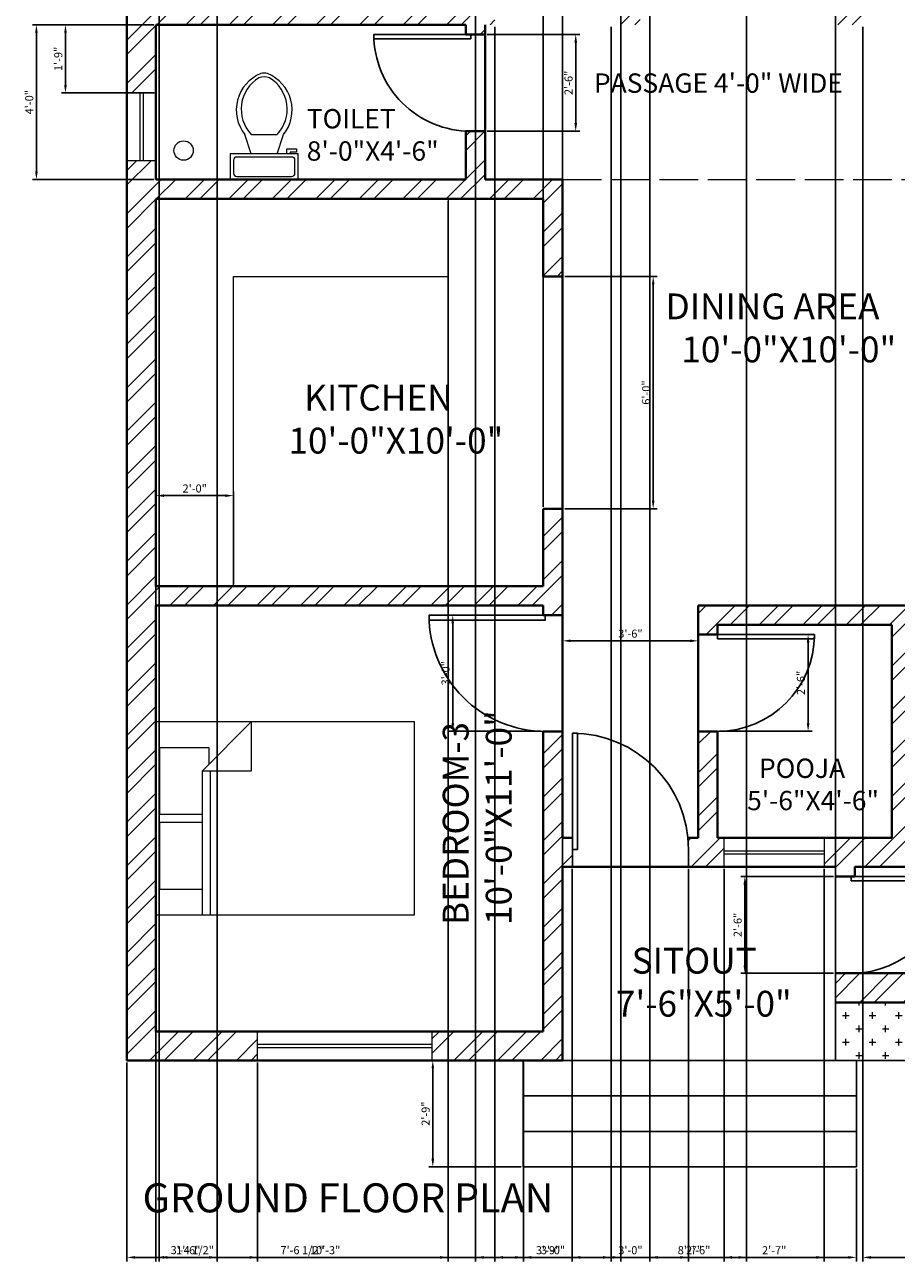
# Model space of a CAD drawing. Units: inches. Extents: x 201 to 622, y 55 to 632.
# Tile 1 of 3: x 201 to 471, y 55 to 439. Entities that reach past the tile are written whole.
import ezdxf

# ---------------------------------------------------------------- set-up
doc = ezdxf.new("R2010")
doc.units = ezdxf.units.IN
doc.linetypes.add('ACAD_ISO02W100', pattern=[15, 12, -3])
for name, color, linetype, lineweight in [('A-ANNO-DIMS', 2, 'Continuous', 18), ('A-ANNO-TITL', 7, 'Continuous', 25), ('A-AREA-IDEN', 7, 'Continuous', 18), ('A-DOOR', 4, 'Continuous', 25), ('A-FLOR', 7, 'Continuous', 25), ('A-FLOR-CASE', 8, 'Continuous', 18), ('A-FLOR-FIXT', 8, 'Continuous', 18), ('A-FLOR-OVHD', 7, 'ACAD_ISO02W100', 18), ('A-FLOR-STRS', 7, 'Continuous', 25), ('A-WALL', 7, 'Continuous', 40), ('A-WALL-PATT', 252, 'Continuous', 13)]:
    doc.layers.add(name, color=color, linetype=linetype, lineweight=lineweight)
for name, color, linetype, lineweight, true_color in [('A-FLOR-PATT', 116, 'Continuous', 13, 0x136734), ('A-FURN', 152, 'Continuous', 18, 0x2776bb), ('A-GLAZ', 152, 'Continuous', 18, 0x2776bb)]:
    doc.layers.add(name, color=color, linetype=linetype, lineweight=lineweight, true_color=true_color)
doc.styles.get("Standard").update_dxf_attribs({"font": 'arial.ttf'})
doc.dimstyles.new('ISO-25', dxfattribs={"dimtxt": 2.5, "dimasz": 2.5, "dimexe": 1.25, "dimexo": 0.625, "dimtad": 1, "dimlunit": 3, "dimtxsty": 'Standard', "dimcen": 2.5, "dimadec": 0, "dimazin": 0, "dimtfac": 1, "dimtmove": 0, "dimatfit": 3, "dimfxl": 1, "dimarcsym": 0})

# ---------------------------------------------------------------- blocks, each defined once
blk = doc.blocks.new('*U3')
for p, q in [((0, 0), (0, -6)), ((40, 0), (40, -6))]:
    blk.add_line(p, q)
blk.add_lwpolyline([(0, 0), (0, 40), (1.75, 40), (1.75, 0)], close=True)
blk.add_arc((0, 0), 40, 0, 90)
blk = doc.blocks.new('*U5')
for p, q in [((0, 0), (0, 6)), ((40, 0), (40, 6))]:
    blk.add_line(p, q)
blk.add_lwpolyline([(0, 0), (0, -40), (1.75, -40), (1.75, 0)], close=True)
blk.add_arc((0, 0), 40, 270, 0)
blk = doc.blocks.new('*U6')
for p, q in [((0, 0), (0, -6)), ((40, 0), (40, -6))]:
    blk.add_line(p, q)
blk.add_lwpolyline([(0, 0), (0, 40), (1.75, 40), (1.75, 0)], close=True)
blk.add_arc((0, 0), 40, 0, 90)
blk = doc.blocks.new('Bed - Queen')
for p, q in [((0, -80.00003), (0, 0)), ((0, 0), (59.99999, 0)), ((59.99999, 0), (59.99999, -80.00003)), ((7.99999, -1.2), (28.79998, -1.2)), ((7.99999, -14.4), (7.99999, -1.2)), ((28.79998, -1.2), (28.79998, -14.4)), ((31.19999, -1.2), (51.99999, -1.2)), ((31.19999, -14.4), (31.19999, -1.2)), ((51.99999, -1.2), (51.99999, -16.4)), ((0, -14.4), (44.8, -14.4)), ((59.99999, -29.6), (44.8, -14.4)), ((44.8, -14.4), (44.8, -29.6)), ((44.8, -16.8), (0, -16.8)), ((51.99999, -16.4), (46.79936, -16.4)), ((44.8, -29.6), (59.99999, -29.6)), ((59.99999, -80.00003), (0, -80.00003))]:
    blk.add_line(p, q)
blk = doc.blocks.new('*U9')
for p, q in [((9.5, -6), (9.5, -2)), ((-10, -8.5), (-8, -8.5)), ((-10, -9.5), (-10, -8.5)), ((-7, -9.5), (-10, -9.5)), ((-8, -8.5), (-8, -8)), ((-7, -8), (-7, -9.5)), ((-4, -8), (-6, -14)), ((4, -8), (6, -14)), ((4, -14), (-4, -14))]:
    blk.add_line(p, q)
blk.add_lwpolyline([(10.5, -8), (10.5, 0), (-10.5, 0), (-10.5, -8)], close=True)
for points in [[(-9.5, -2), (-9.5, -6)], [(8.5, -1), (-8.5, -1)], [(-8.5, -7), (8.5, -7)]]:
    blk.add_lwpolyline(points)
for centre, radius, start, end in [((-8.62, -1.88), 0.884, 81.8699, 188.1301), ((8.62, -1.88), 0.884, 351.8699, 98.1301), ((-8.62, -6.12), 0.884, 171.8699, 278.1301), ((8.62, -6.12), 0.884, 261.8699, 8.1301), ((3.52, -21.58), 12.17, 141.4691, 247.9714), ((4.2, -21.82), 11.33, 136.3677, 238.9468), ((-3.52, -21.58), 12.17, 292.0284, 38.5307), ((-4.2, -21.82), 11.33, 301.053, 43.6321), ((0, -27.88), 4, 245.7318, 294.2682), ((0, -29), 4, 254.8605, 285.1395)]:
    blk.add_arc(centre, radius, start, end)
blk = doc.blocks.new('WIN-54')
for p, q in [((0, 5), (54, 5)), ((0, 4), (54, 4))]:
    blk.add_line(p, q)
blk.add_lwpolyline([(0, 9), (54, 9), (54, 0), (0, 0)], close=True)
blk = doc.blocks.new('WIN-21')
for p, q in [((0, 5), (21, 5)), ((0, 4), (21, 4))]:
    blk.add_line(p, q)
blk.add_lwpolyline([(0, 0), (0, 9), (21, 9), (21, 0)], close=True)
blk = doc.blocks.new('*D23')
at = {"layer": 'A-ANNO-DIMS', "color": 0, "lineweight": -2, "transparency": 16777216}
for p, q in [((354.55, 118.15), (325.88, 118.15)), ((327.13, 87.65), (327.13, 115.65)), ((354.55, 85.15), (325.88, 85.15))]:
    blk.add_line(p, q, dxfattribs=at)
at = {"layer": 'A-ANNO-DIMS', "color": 0, "transparency": 16777216}
for points in [[(326.71, 115.65), (327.54, 115.65), (327.13, 118.15)], [(326.71, 87.65), (327.54, 87.65), (327.13, 85.15)]]:
    blk.add_solid(points, dxfattribs=at)
at = {"layer": 'Defpoints', "color": 0, "transparency": 16777216}
for p in [(327.13, 118.15), (355.18, 118.15), (355.18, 85.15)]:
    blk.add_point(p, dxfattribs=at)
at = {"layer": 'A-ANNO-DIMS', "color": 0, "transparency": 16777216, "insert": (325.22, 101.65), "char_height": 2.5, "attachment_point": 5, "rotation": 90}
blk.add_mtext('2\'-9"', dxfattribs=at)
blk = doc.blocks.new('*D24')
at = {"layer": 'A-ANNO-DIMS', "color": 0, "lineweight": -2, "transparency": 16777216}
for p, q in [((355.18, 84.52), (355.18, 55.85)), ((458.38, 84.52), (458.38, 55.85)), ((357.68, 57.1), (455.88, 57.1))]:
    blk.add_line(p, q, dxfattribs=at)
at = {"layer": 'A-ANNO-DIMS', "color": 0, "transparency": 16777216}
for points in [[(357.68, 57.51), (357.68, 56.68), (355.18, 57.1)], [(455.88, 57.51), (455.88, 56.68), (458.38, 57.1)]]:
    blk.add_solid(points, dxfattribs=at)
at = {"layer": 'Defpoints', "color": 0, "transparency": 16777216}
for p in [(355.18, 85.15), (458.38, 85.15), (458.38, 57.1)]:
    blk.add_point(p, dxfattribs=at)
at = {"layer": 'A-ANNO-DIMS', "color": 0, "transparency": 16777216, "insert": (406.78, 59), "char_height": 2.5, "attachment_point": 5}
blk.add_mtext('8\'-7"', dxfattribs=at)
blk = doc.blocks.new('*D25')
at = {"layer": 'A-ANNO-DIMS', "color": 0, "lineweight": -2, "transparency": 16777216}
for p, q in [((232.36, 117.52), (232.36, 55.85)), ((355.18, 117.52), (355.18, 55.85)), ((234.86, 57.1), (352.68, 57.1))]:
    blk.add_line(p, q, dxfattribs=at)
at = {"layer": 'A-ANNO-DIMS', "color": 0, "transparency": 16777216}
for points in [[(234.86, 57.51), (234.86, 56.68), (232.36, 57.1)], [(352.68, 57.51), (352.68, 56.68), (355.18, 57.1)]]:
    blk.add_solid(points, dxfattribs=at)
at = {"layer": 'Defpoints', "color": 0, "transparency": 16777216}
for p in [(232.36, 118.15), (355.18, 118.15), (355.18, 57.1)]:
    blk.add_point(p, dxfattribs=at)
at = {"layer": 'A-ANNO-DIMS', "color": 0, "transparency": 16777216, "insert": (293.77, 59), "char_height": 2.5, "attachment_point": 5}
blk.add_mtext('10\'-3"', dxfattribs=at)
blk = doc.blocks.new('*D27')
at = {"layer": 'A-ANNO-DIMS', "color": 0, "lineweight": -2, "transparency": 16777216}
for p, q in [((358.86, 626.2), (356.36, 626.2)), ((361.36, 289.77), (361.36, 627.45)), ((361.36, 626.2), (367.36, 626.2)), ((367.36, 289.77), (367.36, 627.45)), ((369.86, 626.2), (380.26, 626.2))]:
    blk.add_line(p, q, dxfattribs=at)
at = {"layer": 'A-ANNO-DIMS', "color": 0, "transparency": 16777216}
for points in [[(358.86, 626.61), (358.86, 625.78), (361.36, 626.2)], [(369.86, 626.61), (369.86, 625.78), (367.36, 626.2)]]:
    blk.add_solid(points, dxfattribs=at)
at = {"layer": 'Defpoints', "color": 0, "transparency": 16777216}
for p in [(367.36, 626.2), (361.36, 289.15), (367.36, 289.15)]:
    blk.add_point(p, dxfattribs=at)
at = {"layer": 'A-ANNO-DIMS', "color": 0, "transparency": 16777216, "insert": (376.31, 628.1), "char_height": 2.5, "attachment_point": 5}
blk.add_mtext('0\'-6"', dxfattribs=at)
blk = doc.blocks.new('*D28')
at = {"layer": 'A-ANNO-DIMS', "color": 0, "lineweight": -2, "transparency": 16777216}
for p, q in [((367.99, 361.15), (396.66, 361.15)), ((395.41, 358.65), (395.41, 291.65)), ((367.99, 289.15), (396.66, 289.15))]:
    blk.add_line(p, q, dxfattribs=at)
at = {"layer": 'A-ANNO-DIMS', "color": 0, "transparency": 16777216}
for points in [[(395, 358.65), (395.83, 358.65), (395.41, 361.15)], [(395, 291.65), (395.83, 291.65), (395.41, 289.15)]]:
    blk.add_solid(points, dxfattribs=at)
at = {"layer": 'Defpoints', "color": 0, "transparency": 16777216}
for p in [(367.36, 361.15), (367.36, 289.15), (395.41, 289.15)]:
    blk.add_point(p, dxfattribs=at)
at = {"layer": 'A-ANNO-DIMS', "color": 0, "transparency": 16777216, "insert": (393.51, 325.15), "char_height": 2.5, "attachment_point": 5, "rotation": 90}
blk.add_mtext('6\'-0"', dxfattribs=at)
blk = doc.blocks.new('*D29')
at = {"layer": 'A-ANNO-DIMS', "color": 0, "lineweight": -2, "transparency": 16777216}
for p, q in [((340.36, 588.52), (340.36, 55.85)), ((385.36, 588.52), (385.36, 55.85)), ((342.86, 57.1), (382.86, 57.1))]:
    blk.add_line(p, q, dxfattribs=at)
at = {"layer": 'A-ANNO-DIMS', "color": 0, "transparency": 16777216}
for points in [[(342.86, 57.51), (342.86, 56.68), (340.36, 57.1)], [(382.86, 57.51), (382.86, 56.68), (385.36, 57.1)]]:
    blk.add_solid(points, dxfattribs=at)
at = {"layer": 'Defpoints', "color": 0, "transparency": 16777216}
for p in [(340.36, 589.15), (385.36, 589.15), (385.36, 57.1)]:
    blk.add_point(p, dxfattribs=at)
at = {"layer": 'A-ANNO-DIMS', "color": 0, "transparency": 16777216, "insert": (362.86, 59), "char_height": 2.5, "attachment_point": 5}
blk.add_mtext('3\'-9"', dxfattribs=at)
blk = doc.blocks.new('*D35')
at = {"layer": 'A-ANNO-DIMS', "color": 0, "lineweight": -2, "transparency": 16777216}
for p, q in [((232.36, 117.52), (232.36, 55.85)), ((272.86, 117.52), (272.86, 55.85)), ((234.86, 57.1), (270.36, 57.1))]:
    blk.add_line(p, q, dxfattribs=at)
at = {"layer": 'A-ANNO-DIMS', "color": 0, "transparency": 16777216}
for points in [[(234.86, 57.51), (234.86, 56.68), (232.36, 57.1)], [(270.36, 57.51), (270.36, 56.68), (272.86, 57.1)]]:
    blk.add_solid(points, dxfattribs=at)
at = {"layer": 'Defpoints', "color": 0, "transparency": 16777216}
for p in [(232.36, 118.15), (272.86, 118.15), (272.86, 57.1)]:
    blk.add_point(p, dxfattribs=at)
at = {"layer": 'A-ANNO-DIMS', "color": 0, "transparency": 16777216, "insert": (252.61, 59.02), "char_height": 2.5, "attachment_point": 5}
blk.add_mtext('3\'-4 1/2"', dxfattribs=at)
blk = doc.blocks.new('*D37')
at = {"layer": 'A-ANNO-DIMS', "color": 0, "lineweight": -2, "transparency": 16777216}
for p, q in [((240.74, 439.15), (212.06, 439.15)), ((213.31, 420.5), (213.31, 436.65)), ((240.74, 418), (212.06, 418))]:
    blk.add_line(p, q, dxfattribs=at)
at = {"layer": 'A-ANNO-DIMS', "color": 0, "transparency": 16777216}
for points in [[(212.9, 436.65), (213.73, 436.65), (213.31, 439.15)], [(212.9, 420.5), (213.73, 420.5), (213.31, 418)]]:
    blk.add_solid(points, dxfattribs=at)
at = {"layer": 'Defpoints', "color": 0, "transparency": 16777216}
for p in [(213.31, 439.15), (241.36, 439.15), (241.36, 418)]:
    blk.add_point(p, dxfattribs=at)
at = {"layer": 'A-ANNO-DIMS', "color": 0, "transparency": 16777216, "insert": (211.41, 428.57), "char_height": 2.5, "attachment_point": 5, "rotation": 90}
blk.add_mtext('1\'-9"', dxfattribs=at)
blk = doc.blocks.new('*D38')
at = {"layer": 'A-ANNO-DIMS', "color": 0, "lineweight": -2, "transparency": 16777216}
for p, q in [((370.36, 177.52), (370.36, 55.85)), ((406.36, 177.52), (406.36, 55.85)), ((372.86, 57.1), (403.86, 57.1))]:
    blk.add_line(p, q, dxfattribs=at)
at = {"layer": 'A-ANNO-DIMS', "color": 0, "transparency": 16777216}
for points in [[(372.86, 57.51), (372.86, 56.68), (370.36, 57.1)], [(403.86, 57.51), (403.86, 56.68), (406.36, 57.1)]]:
    blk.add_solid(points, dxfattribs=at)
at = {"layer": 'Defpoints', "color": 0, "transparency": 16777216}
for p in [(370.36, 178.15), (406.36, 178.15), (406.36, 57.1)]:
    blk.add_point(p, dxfattribs=at)
at = {"layer": 'A-ANNO-DIMS', "color": 0, "transparency": 16777216, "insert": (388.36, 59), "char_height": 2.5, "attachment_point": 5}
blk.add_mtext('3\'-0"', dxfattribs=at)
blk = doc.blocks.new('*D39')
at = {"layer": 'A-ANNO-DIMS', "color": 0, "lineweight": -2, "transparency": 16777216}
for p, q in [((346.36, 438.52), (346.36, 55.85)), ((382.36, 438.52), (382.36, 55.85)), ((348.86, 57.1), (379.86, 57.1))]:
    blk.add_line(p, q, dxfattribs=at)
at = {"layer": 'A-ANNO-DIMS', "color": 0, "transparency": 16777216}
for points in [[(348.86, 57.51), (348.86, 56.68), (346.36, 57.1)], [(379.86, 57.51), (379.86, 56.68), (382.36, 57.1)]]:
    blk.add_solid(points, dxfattribs=at)
at = {"layer": 'Defpoints', "color": 0, "transparency": 16777216}
for p in [(346.36, 439.15), (382.36, 439.15), (382.36, 57.1)]:
    blk.add_point(p, dxfattribs=at)
at = {"layer": 'A-ANNO-DIMS', "color": 0, "transparency": 16777216, "insert": (364.36, 59), "char_height": 2.5, "attachment_point": 5}
blk.add_mtext('3\'-0"', dxfattribs=at)
blk = doc.blocks.new('*D40')
at = {"layer": 'A-ANNO-DIMS', "color": 0, "lineweight": -2, "transparency": 16777216}
for p, q in [((394.36, 486.52), (394.36, 55.85)), ((424.36, 486.52), (424.36, 55.85)), ((396.86, 57.1), (421.86, 57.1))]:
    blk.add_line(p, q, dxfattribs=at)
at = {"layer": 'A-ANNO-DIMS', "color": 0, "transparency": 16777216}
for points in [[(396.86, 57.51), (396.86, 56.68), (394.36, 57.1)], [(421.86, 57.51), (421.86, 56.68), (424.36, 57.1)]]:
    blk.add_solid(points, dxfattribs=at)
at = {"layer": 'Defpoints', "color": 0, "transparency": 16777216}
for p in [(394.36, 487.15), (424.36, 487.15), (424.36, 57.1)]:
    blk.add_point(p, dxfattribs=at)
at = {"layer": 'A-ANNO-DIMS', "color": 0, "transparency": 16777216, "insert": (409.36, 59), "char_height": 2.5, "attachment_point": 5}
blk.add_mtext('2\'-6"', dxfattribs=at)
blk = doc.blocks.new('*D42')
at = {"layer": 'A-ANNO-DIMS', "color": 0, "lineweight": -2, "transparency": 16777216}
for p, q in [((241.36, 265.77), (241.36, 294.45)), ((243.86, 293.2), (262.86, 293.2)), ((265.36, 265.77), (265.36, 294.45))]:
    blk.add_line(p, q, dxfattribs=at)
at = {"layer": 'A-ANNO-DIMS', "color": 0, "transparency": 16777216}
for points in [[(243.86, 293.61), (243.86, 292.78), (241.36, 293.2)], [(262.86, 293.61), (262.86, 292.78), (265.36, 293.2)]]:
    blk.add_solid(points, dxfattribs=at)
at = {"layer": 'Defpoints', "color": 0, "transparency": 16777216}
for p in [(265.36, 293.2), (241.36, 265.15), (265.36, 265.15)]:
    blk.add_point(p, dxfattribs=at)
at = {"layer": 'A-ANNO-DIMS', "color": 0, "transparency": 16777216, "insert": (253.36, 295.1), "char_height": 2.5, "attachment_point": 5}
blk.add_mtext('2\'-0"', dxfattribs=at)
blk = doc.blocks.new('*D44')
at = {"layer": 'A-ANNO-DIMS', "color": 0, "lineweight": -2, "transparency": 16777216}
for p, q in [((367.36, 220.77), (367.36, 249.45)), ((369.86, 248.2), (406.86, 248.2)), ((409.36, 220.77), (409.36, 249.45))]:
    blk.add_line(p, q, dxfattribs=at)
at = {"layer": 'A-ANNO-DIMS', "color": 0, "transparency": 16777216}
for points in [[(369.86, 248.61), (369.86, 247.78), (367.36, 248.2)], [(406.86, 248.61), (406.86, 247.78), (409.36, 248.2)]]:
    blk.add_solid(points, dxfattribs=at)
at = {"layer": 'Defpoints', "color": 0, "transparency": 16777216}
for p in [(409.36, 248.2), (367.36, 220.15), (409.36, 220.15)]:
    blk.add_point(p, dxfattribs=at)
at = {"layer": 'A-ANNO-DIMS', "color": 0, "transparency": 16777216, "insert": (388.36, 250.1), "char_height": 2.5, "attachment_point": 5}
blk.add_mtext('3\'-6"', dxfattribs=at)
blk = doc.blocks.new('*D45')
at = {"layer": 'A-ANNO-DIMS', "color": 0, "lineweight": -2, "transparency": 16777216}
for p, q in [((417.38, 177.52), (417.38, 55.85)), ((448.42, 177.52), (448.42, 55.85)), ((419.88, 57.1), (445.92, 57.1))]:
    blk.add_line(p, q, dxfattribs=at)
at = {"layer": 'A-ANNO-DIMS', "color": 0, "transparency": 16777216}
for points in [[(419.88, 57.51), (419.88, 56.68), (417.38, 57.1)], [(445.92, 57.51), (445.92, 56.68), (448.42, 57.1)]]:
    blk.add_solid(points, dxfattribs=at)
at = {"layer": 'Defpoints', "color": 0, "transparency": 16777216}
for p in [(417.38, 178.15), (448.42, 178.15), (448.42, 57.1)]:
    blk.add_point(p, dxfattribs=at)
at = {"layer": 'A-ANNO-DIMS', "color": 0, "transparency": 16777216, "insert": (432.9, 58.98), "char_height": 2.5, "attachment_point": 5}
blk.add_mtext('2\'-7"', dxfattribs=at)
blk = doc.blocks.new('*D47')
at = {"layer": 'A-ANNO-DIMS', "color": 0, "lineweight": -2, "transparency": 16777216}
for p, q in [((240.74, 439.15), (203.06, 439.15)), ((204.31, 393.65), (204.31, 436.65)), ((240.74, 391.15), (203.06, 391.15))]:
    blk.add_line(p, q, dxfattribs=at)
at = {"layer": 'A-ANNO-DIMS', "color": 0, "transparency": 16777216}
for points in [[(203.9, 436.65), (204.73, 436.65), (204.31, 439.15)], [(203.9, 393.65), (204.73, 393.65), (204.31, 391.15)]]:
    blk.add_solid(points, dxfattribs=at)
at = {"layer": 'Defpoints', "color": 0, "transparency": 16777216}
for p in [(204.31, 439.15), (241.36, 439.15), (241.36, 391.15)]:
    blk.add_point(p, dxfattribs=at)
at = {"layer": 'A-ANNO-DIMS', "color": 0, "transparency": 16777216, "insert": (202.41, 415.15), "char_height": 2.5, "attachment_point": 5, "rotation": 90}
blk.add_mtext('4\'-0"', dxfattribs=at)
blk = doc.blocks.new('*D48')
at = {"layer": 'A-ANNO-DIMS', "color": 0, "lineweight": -2, "transparency": 16777216}
for p, q in [((367.36, 118.77), (367.36, 627.45)), ((369.86, 626.2), (449.36, 626.2)), ((451.86, 118.77), (451.86, 627.45))]:
    blk.add_line(p, q, dxfattribs=at)
at = {"layer": 'A-ANNO-DIMS', "color": 0, "transparency": 16777216}
for points in [[(369.86, 626.61), (369.86, 625.78), (367.36, 626.2)], [(449.36, 626.61), (449.36, 625.78), (451.86, 626.2)]]:
    blk.add_solid(points, dxfattribs=at)
at = {"layer": 'Defpoints', "color": 0, "transparency": 16777216}
for p in [(451.86, 626.2), (367.36, 118.15), (451.86, 118.15)]:
    blk.add_point(p, dxfattribs=at)
at = {"layer": 'A-ANNO-DIMS', "color": 0, "transparency": 16777216, "insert": (409.61, 628.11), "char_height": 2.5, "attachment_point": 5}
blk.add_mtext('7\'-0 1/2"', dxfattribs=at)
blk = doc.blocks.new('*D49')
at = {"layer": 'A-ANNO-DIMS', "color": 0, "lineweight": -2, "transparency": 16777216}
for p, q in [((460.36, 438.52), (460.36, 55.85)), ((496.36, 438.52), (496.36, 55.85)), ((462.86, 57.1), (493.86, 57.1))]:
    blk.add_line(p, q, dxfattribs=at)
at = {"layer": 'A-ANNO-DIMS', "color": 0, "transparency": 16777216}
for points in [[(462.86, 57.51), (462.86, 56.68), (460.36, 57.1)], [(493.86, 57.51), (493.86, 56.68), (496.36, 57.1)]]:
    blk.add_solid(points, dxfattribs=at)
at = {"layer": 'Defpoints', "color": 0, "transparency": 16777216}
for p in [(460.36, 439.15), (496.36, 439.15), (496.36, 57.1)]:
    blk.add_point(p, dxfattribs=at)
at = {"layer": 'A-ANNO-DIMS', "color": 0, "transparency": 16777216, "insert": (478.36, 59), "char_height": 2.5, "attachment_point": 5}
blk.add_mtext('3\'-0"', dxfattribs=at)
blk = doc.blocks.new('*D50')
at = {"layer": 'A-ANNO-DIMS', "color": 0, "lineweight": -2, "transparency": 16777216}
for p, q in [((343.99, 436.15), (372.66, 436.15)), ((371.41, 433.65), (371.41, 408.65)), ((343.99, 406.15), (372.66, 406.15))]:
    blk.add_line(p, q, dxfattribs=at)
at = {"layer": 'A-ANNO-DIMS', "color": 0, "transparency": 16777216}
for points in [[(371, 433.65), (371.83, 433.65), (371.41, 436.15)], [(371, 408.65), (371.83, 408.65), (371.41, 406.15)]]:
    blk.add_solid(points, dxfattribs=at)
at = {"layer": 'Defpoints', "color": 0, "transparency": 16777216}
for p in [(343.36, 436.15), (343.36, 406.15), (371.41, 406.15)]:
    blk.add_point(p, dxfattribs=at)
at = {"layer": 'A-ANNO-DIMS', "color": 0, "transparency": 16777216, "insert": (369.51, 421.15), "char_height": 2.5, "attachment_point": 5, "rotation": 90}
blk.add_mtext('2\'-6"', dxfattribs=at)
blk = doc.blocks.new('*D51')
at = {"layer": 'A-ANNO-DIMS', "color": 0, "lineweight": -2, "transparency": 16777216}
for p, q in [((360.74, 256.15), (332.06, 256.15)), ((333.31, 222.65), (333.31, 253.65)), ((360.74, 220.15), (332.06, 220.15))]:
    blk.add_line(p, q, dxfattribs=at)
at = {"layer": 'A-ANNO-DIMS', "color": 0, "transparency": 16777216}
for points in [[(332.9, 253.65), (333.73, 253.65), (333.31, 256.15)], [(332.9, 222.65), (333.73, 222.65), (333.31, 220.15)]]:
    blk.add_solid(points, dxfattribs=at)
at = {"layer": 'Defpoints', "color": 0, "transparency": 16777216}
for p in [(333.31, 256.15), (361.36, 256.15), (361.36, 220.15)]:
    blk.add_point(p, dxfattribs=at)
at = {"layer": 'A-ANNO-DIMS', "color": 0, "transparency": 16777216, "insert": (331.41, 238.15), "char_height": 2.5, "attachment_point": 5, "rotation": 90}
blk.add_mtext('3\'-0"', dxfattribs=at)
blk = doc.blocks.new('*D52')
at = {"layer": 'A-ANNO-DIMS', "color": 0, "lineweight": -2, "transparency": 16777216}
for p, q in [((415.99, 250.15), (444.66, 250.15)), ((443.41, 247.65), (443.41, 222.65)), ((415.99, 220.15), (444.66, 220.15))]:
    blk.add_line(p, q, dxfattribs=at)
at = {"layer": 'A-ANNO-DIMS', "color": 0, "transparency": 16777216}
for points in [[(443, 247.65), (443.83, 247.65), (443.41, 250.15)], [(443, 222.65), (443.83, 222.65), (443.41, 220.15)]]:
    blk.add_solid(points, dxfattribs=at)
at = {"layer": 'Defpoints', "color": 0, "transparency": 16777216}
for p in [(415.36, 250.15), (415.36, 220.15), (443.41, 220.15)]:
    blk.add_point(p, dxfattribs=at)
at = {"layer": 'A-ANNO-DIMS', "color": 0, "transparency": 16777216, "insert": (441.51, 235.15), "char_height": 2.5, "attachment_point": 5, "rotation": 90}
blk.add_mtext('2\'-6"', dxfattribs=at)
blk = doc.blocks.new('*D53')
at = {"layer": 'A-ANNO-DIMS', "color": 0, "lineweight": -2, "transparency": 16777216}
for p, q in [((451.23, 175.15), (422.56, 175.15)), ((423.81, 147.65), (423.81, 172.65)), ((451.23, 145.15), (422.56, 145.15))]:
    blk.add_line(p, q, dxfattribs=at)
at = {"layer": 'A-ANNO-DIMS', "color": 0, "transparency": 16777216}
for points in [[(423.39, 172.65), (424.22, 172.65), (423.81, 175.15)], [(423.39, 147.65), (424.22, 147.65), (423.81, 145.15)]]:
    blk.add_solid(points, dxfattribs=at)
at = {"layer": 'Defpoints', "color": 0, "transparency": 16777216}
for p in [(423.81, 175.15), (451.86, 175.15), (451.86, 145.15)]:
    blk.add_point(p, dxfattribs=at)
at = {"layer": 'A-ANNO-DIMS', "color": 0, "transparency": 16777216, "insert": (421.91, 160.15), "char_height": 2.5, "attachment_point": 5, "rotation": 90}
blk.add_mtext('2\'-6"', dxfattribs=at)
blk = doc.blocks.new('*D56')
at = {"layer": 'A-ANNO-DIMS', "color": 0, "lineweight": -2, "transparency": 16777216}
for p, q in [((242.36, 527.98), (242.36, 55.85)), ((260.36, 527.98), (260.36, 55.85)), ((244.86, 57.1), (257.86, 57.1))]:
    blk.add_line(p, q, dxfattribs=at)
at = {"layer": 'A-ANNO-DIMS', "color": 0, "transparency": 16777216}
for points in [[(244.86, 57.51), (244.86, 56.68), (242.36, 57.1)], [(257.86, 57.51), (257.86, 56.68), (260.36, 57.1)]]:
    blk.add_solid(points, dxfattribs=at)
at = {"layer": 'Defpoints', "color": 0, "transparency": 16777216}
for p in [(242.36, 528.6), (260.36, 528.6), (260.36, 57.1)]:
    blk.add_point(p, dxfattribs=at)
at = {"layer": 'A-ANNO-DIMS', "color": 0, "transparency": 16777216, "insert": (251.36, 59), "char_height": 2.5, "attachment_point": 5}
blk.add_mtext('1\'-6"', dxfattribs=at)
blk = doc.blocks.new('*D58')
at = {"layer": 'A-ANNO-DIMS', "color": 0, "lineweight": -2, "transparency": 16777216}
for p, q in [((241.36, 384.52), (241.36, 55.85)), ((331.89, 384.52), (331.89, 55.85)), ((243.86, 57.1), (329.39, 57.1))]:
    blk.add_line(p, q, dxfattribs=at)
at = {"layer": 'A-ANNO-DIMS', "color": 0, "transparency": 16777216}
for points in [[(243.86, 57.51), (243.86, 56.68), (241.36, 57.1)], [(329.39, 57.51), (329.39, 56.68), (331.89, 57.1)]]:
    blk.add_solid(points, dxfattribs=at)
at = {"layer": 'Defpoints', "color": 0, "transparency": 16777216}
for p in [(241.36, 385.15), (331.89, 385.15), (331.89, 57.1)]:
    blk.add_point(p, dxfattribs=at)
at = {"layer": 'A-ANNO-DIMS', "color": 0, "transparency": 16777216, "insert": (286.63, 59.01), "char_height": 2.5, "attachment_point": 5}
blk.add_mtext('7\'-6 1/2"', dxfattribs=at)

msp = doc.modelspace()

# ---------------------------------------------------------------- hatches: boundary and pattern name
at = {"layer": 'A-FLOR-PATT'}
h = msp.add_hatch(dxfattribs=at)
h.set_pattern_fill('CROSS', color=256, scale=0.65)
h.paths.add_polyline_path([(592.362, 136.147), (451.858, 136.147), (451.858, 118.147), (592.362, 118.147)])
at = {"layer": 'A-WALL-PATT'}
h = msp.add_hatch(dxfattribs=at)
h.set_pattern_fill('ANSI32', color=256)
h.paths.add_polyline_path([(241.362, 589.147), (286.362, 589.147), (286.362, 598.147), (232.362, 598.147), (232.362, 418.002), (241.362, 418.002), (241.362, 439.147), (337.362, 439.147), (337.362, 436.147), (343.362, 436.147), (343.362, 439.147), (346.362, 439.147), (346.362, 445.147), (241.362, 445.147)])
h.paths.add_polyline_path([(394.362, 493.147), (391.362, 493.147), (391.362, 589.147), (426.354, 589.147), (426.354, 598.147), (340.362, 598.147), (340.362, 589.147), (385.362, 589.147), (385.362, 445.147), (382.362, 445.147), (382.362, 439.147), (391.362, 439.147), (391.362, 487.147), (394.362, 487.147)])
h.paths.add_polyline_path([(457.362, 589.147), (493.362, 589.147), (493.362, 598.147), (447.354, 598.147), (447.354, 589.147), (451.362, 589.147), (451.362, 493.147), (424.362, 493.147), (424.362, 487.147), (451.362, 487.147), (451.362, 439.147), (460.362, 439.147), (460.362, 445.147), (457.362, 445.147)])
h.paths.add_polyline_path([(592.362, 598.147), (547.362, 598.147), (547.362, 589.147), (550.362, 589.147), (583.362, 589.147), (583.362, 544.147), (592.362, 544.147)])
h.paths.add_polyline_path([(592.362, 490.147), (583.362, 490.147), (583.362, 445.147), (496.362, 445.147), (496.362, 439.147), (583.362, 439.147), (583.362, 406.147), (592.362, 406.147)])
h.paths.add_polyline_path([(592.362, 352.147), (583.362, 352.147), (583.362, 319.147), (532.362, 319.147), (532.362, 313.147), (583.362, 313.147), (583.362, 256.147), (592.362, 256.147)])
h.paths.add_polyline_path([(592.362, 202.147), (583.362, 202.147), (583.362, 145.147), (549.11, 145.147), (549.11, 136.147), (592.362, 136.147)])
h.paths.add_polyline_path([(493.362, 313.147), (496.362, 313.147), (496.362, 319.147), (487.362, 319.147), (487.362, 259.147), (409.362, 259.147), (409.362, 250.147), (415.362, 250.147), (415.362, 253.147), (469.362, 253.147), (469.362, 187.147), (448.415, 187.147), (448.415, 178.147), (451.858, 178.147), (451.858, 175.147), (457.858, 175.147), (457.858, 178.147), (475.362, 178.147), (475.362, 253.147), (493.362, 253.147)])
h.paths.add_polyline_path([(495.11, 145.147), (457.858, 145.147), (451.858, 145.147), (451.858, 136.147), (495.11, 136.147)])
h.paths.add_polyline_path([(367.362, 178.147), (370.362, 178.147), (370.362, 183.547), (370.362, 187.147), (367.362, 187.147), (367.362, 220.147), (361.362, 220.147), (361.362, 127.147), (326.862, 127.147), (326.862, 118.147), (367.362, 118.147)])
h.paths.add_polyline_path([(272.862, 127.147), (241.362, 127.147), (241.362, 259.147), (361.362, 259.147), (361.362, 256.147), (361.962, 256.147), (367.362, 256.147), (367.362, 289.147), (361.362, 289.147), (361.362, 265.147), (241.362, 265.147), (241.362, 385.147), (361.362, 385.147), (361.362, 361.147), (367.362, 361.147), (367.362, 391.147), (343.362, 391.147), (343.362, 406.147), (338.862, 406.147), (337.362, 406.147), (337.362, 391.147), (241.362, 391.147), (241.362, 397.002), (232.362, 397.002), (232.362, 118.147), (272.862, 118.147)])
h.paths.add_polyline_path([(417.381, 187.147), (415.362, 187.147), (415.362, 220.147), (410.862, 220.147), (409.362, 220.147), (409.362, 187.147), (406.181, 187.147, -0.0250471), (406.362, 183.547), (406.362, 178.147), (417.381, 178.147)])

# ---------------------------------------------------------------- linework, layer by layer
at = {"layer": 'A-FLOR'}
for p, q in [((451.858, 178.147), (451.858, 118.147)), ((592.362, 118.147), (367.362, 118.147))]:
    msp.add_line(p, q, dxfattribs=at)
at = {"layer": 'A-FLOR-CASE'}
for p, q in [((331.889, 385.147), (331.889, 361.147)), ((265.362, 265.147), (265.362, 361.147)), ((265.362, 361.147), (331.889, 361.147))]:
    msp.add_line(p, q, dxfattribs=at)
at = {"layer": 'A-FLOR-FIXT'}
msp.add_circle((249.916, 400.166), 3, dxfattribs=at)
at = {"layer": 'A-FLOR-OVHD'}
msp.add_line((367.362, 391.147), (487.362, 391.147), dxfattribs=at)
at = {"layer": 'A-FLOR-STRS'}
for p, q in [((355.176, 118.147), (355.176, 85.147)), ((458.377, 118.147), (458.377, 85.147)), ((458.377, 107.147), (355.176, 107.147)), ((458.377, 96.147), (355.176, 96.147)), ((458.377, 85.147), (355.176, 85.147))]:
    msp.add_line(p, q, dxfattribs=at)
at = {"layer": 'A-GLAZ'}
for p, q in [((417.381, 183.147), (448.415, 183.147)), ((417.381, 182.147), (448.415, 182.147))]:
    msp.add_line(p, q, dxfattribs=at)
msp.add_lwpolyline([(417.381, 178.147), (417.381, 187.147), (448.415, 187.147), (448.415, 178.147)], close=True, dxfattribs=at)
at = {"layer": 'A-WALL'}
for p, q in [((232.362, 118.147), (232.362, 598.147)), ((241.362, 439.147), (337.362, 439.147)), ((241.362, 391.147), (241.362, 439.147)), ((337.362, 436.147), (337.362, 439.147)), ((343.362, 391.147), (343.362, 439.147)), ((337.362, 436.147), (343.362, 436.147)), ((337.362, 391.147), (337.362, 406.147)), ((337.362, 406.147), (343.362, 406.147)), ((241.362, 391.147), (337.362, 391.147)), ((343.362, 391.147), (367.362, 391.147)), ((367.362, 187.147), (367.362, 391.147)), ((241.362, 385.147), (361.362, 385.147)), ((241.362, 265.147), (241.362, 385.147)), ((361.362, 361.147), (361.362, 385.147)), ((361.362, 361.147), (367.362, 361.147)), ((361.362, 265.147), (361.362, 289.147)), ((361.362, 289.147), (367.362, 289.147)), ((241.362, 265.147), (361.362, 265.147)), ((241.362, 127.147), (241.362, 259.147)), ((241.362, 259.147), (361.362, 259.147)), ((361.362, 256.147), (361.362, 259.147)), ((409.362, 187.147), (409.362, 259.147)), ((409.362, 259.147), (487.362, 259.147)), ((361.362, 256.147), (367.362, 256.147)), ((415.362, 250.147), (409.362, 250.147)), ((415.362, 253.147), (469.362, 253.147)), ((415.362, 250.147), (415.362, 253.147)), ((469.362, 187.147), (469.362, 253.147)), ((361.362, 127.147), (361.362, 220.147)), ((361.362, 220.147), (367.362, 220.147)), ((415.362, 220.147), (409.362, 220.147)), ((415.362, 187.147), (415.362, 220.147)), ((367.362, 187.147), (370.362, 187.147)), ((406.362, 187.147), (409.362, 187.147)), ((415.362, 187.147), (469.362, 187.147)), ((367.362, 118.147), (367.362, 178.147)), ((367.362, 178.147), (451.858, 178.147)), ((457.858, 178.147), (457.858, 175.147)), ((457.858, 178.147), (475.362, 178.147)), ((457.858, 175.147), (451.858, 175.147)), ((457.858, 145.147), (451.858, 145.147)), ((457.858, 145.147), (583.362, 145.147)), ((451.858, 136.147), (592.362, 136.147)), ((361.362, 127.147), (241.362, 127.147)), ((367.362, 118.147), (232.362, 118.147))]:
    msp.add_line(p, q, dxfattribs=at)

# ---------------------------------------------------------------- block references
at = {"layer": 'A-DOOR', "rotation": 270}
for name, p, xscale, yscale, zscale in [('*U5', (338.862, 436.147), 0.75, 0.75, 0.75), ('*U5', (361.962, 256.147), 0.9, 0.9, 0.9), ('*U6', (415.362, 250.147), 0.75, 0.75, 0.75), ('*U6', (456.779, 175.147), 0.75, 0.75, 0.75)]:
    msp.add_blockref(name, p, dxfattribs=dict(at, xscale=xscale, yscale=yscale, zscale=zscale))
at = {"layer": 'A-DOOR', "xscale": 0.9, "yscale": 0.9, "zscale": 0.9}
msp.add_blockref('*U3', (370.362, 183.547), dxfattribs=at)
at = {"layer": 'A-FLOR-FIXT', "rotation": 180}
msp.add_blockref('*U9', (274.891, 391.147), dxfattribs=at)
at = {"layer": 'A-FURN', "rotation": 90}
msp.add_blockref('Bed - Queen', (241.362, 163.147), dxfattribs=at)
at = {"layer": 'A-GLAZ', "rotation": 269.9999999999995}
msp.add_blockref('WIN-21', (232.361, 418.003), dxfattribs=at)
at = {"layer": 'A-GLAZ'}
msp.add_blockref('WIN-54', (272.862, 118.147), dxfattribs=at)

# ---------------------------------------------------------------- texts
at = {"layer": 'A-ANNO-TITL', "insert": (237.199, 80.051), "char_height": 9, "attachment_point": 1}
msp.add_mtext_dynamic_manual_height_columns('GROUND FLOOR PLAN', width=146.12045, gutter_width=12.5, heights=[0], dxfattribs=at)
at = {"layer": 'A-AREA-IDEN', "attachment_point": 1}
for s, width, insert, char_height in [('PASSAGE 4\'-0" WIDE', 84.22071, (377.054, 424.067), 6), ('TOILET\\P8\'-0"X4\'-6"', 38.71373, (288.079, 413.024), 6), ('DINING AREA      10\'-0"X10\'-0"', 74.40783, (399.239, 355.855), 8), ('  KITCHEN\\P10\'-0"X10\'-0"', 68.77314, (282.394, 327.58), 8), ('  POOJA\\P5\'-6"X4\'-6"', 38.71373, (424.524, 211.703), 6), ('  SITOUT        7\'-6"X5\'-0"', 51.04896, (383.859, 153.055), 8)]:
    msp.add_mtext_dynamic_manual_height_columns(s, width=width, gutter_width=12.5, heights=[0], dxfattribs=dict(at, insert=insert, char_height=char_height))
at = {"layer": 'A-AREA-IDEN', "insert": (330.217, 160.104), "char_height": 8, "attachment_point": 1, "rotation": 90}
msp.add_mtext_dynamic_manual_height_columns('BEDROOM-3\\P10\'-0"X11\'-0"', width=68.77314, gutter_width=12.5, heights=[0], dxfattribs=at)

# ---------------------------------------------------------------- dimensions: what is measured, and where the dimension line sits
at = {"layer": 'A-ANNO-DIMS'}
for base, p1, p2, picture, middle in [((367.362, 626.197), (361.362, 289.147), (367.362, 289.147), '*D27', (376.31, 628.099)), ((451.858, 626.197), (367.362, 118.147), (451.858, 118.147), '*D48', (409.61, 628.115)), ((385.362, 57.097), (340.362, 589.147), (385.362, 589.147), '*D29', (362.862, 59)), ((260.362, 57.097), (242.362, 528.603), (260.362, 528.603), '*D56', (251.362, 58.999)), ((424.362, 57.097), (394.362, 487.147), (424.362, 487.147), '*D40', (409.362, 58.999)), ((382.362, 57.097), (346.362, 439.147), (382.362, 439.147), '*D39', (364.362, 59)), ((496.362, 57.097), (460.362, 439.147), (496.362, 439.147), '*D49', (478.362, 59)), ((331.889, 57.097), (241.362, 385.147), (331.889, 385.147), '*D58', (286.626, 59.015)), ((265.362, 293.197), (241.362, 265.147), (265.362, 265.147), '*D42', (253.362, 295.099)), ((409.362, 248.197), (367.362, 220.147), (409.362, 220.147), '*D44', (388.362, 250.1)), ((406.362, 57.097), (370.362, 178.147), (406.362, 178.147), '*D38', (388.362, 59)), ((448.415, 57.097), (417.381, 178.147), (448.415, 178.147), '*D45', (432.898, 58.977)), ((355.176, 57.097), (232.362, 118.147), (355.176, 118.147), '*D25', (293.769, 59)), ((272.862, 57.097), (232.362, 118.147), (272.862, 118.147), '*D35', (252.612, 59.016)), ((458.377, 57.097), (355.176, 85.147), (458.377, 85.147), '*D24', (406.777, 58.999))]:
    dim = msp.add_linear_dim(base=base, p1=p1, p2=p2, dimstyle='ISO-25', override={"dimdec": 1, "dimlfac": 1, "dimrnd": 0, "dimzin": 1, "dimdsep": 46, "dimlunit": 4, "dimfrac": 2}, dxfattribs=at)
    dim.commit()
    dim.dimension.update_dxf_attribs({"geometry": picture, "text_midpoint": middle})
for base, p1, p2, angle, picture, middle in [((204.312, 439.147), (241.362, 391.147), (241.362, 439.147), 90, '*D47', (202.41, 415.147)), ((213.312, 439.147), (241.362, 418.002), (241.362, 439.147), 90, '*D37', (211.41, 428.575)), ((371.412, 406.147), (343.362, 436.147), (343.362, 406.147), 270, '*D50', (369.51, 421.147)), ((395.412, 289.147), (367.362, 361.147), (367.362, 289.147), 270, '*D28', (393.51, 325.147)), ((333.312, 256.147), (361.362, 220.147), (361.362, 256.147), 90, '*D51', (331.41, 238.147)), ((443.412, 220.147), (415.362, 250.147), (415.362, 220.147), 270, '*D52', (441.51, 235.147)), ((423.808, 175.147), (451.858, 145.147), (451.858, 175.147), 90, '*D53', (421.906, 160.147)), ((327.126, 118.147), (355.176, 85.147), (355.176, 118.147), 90, '*D23', (325.225, 101.647))]:
    dim = msp.add_linear_dim(base=base, p1=p1, p2=p2, angle=angle, dimstyle='ISO-25', override={"dimdec": 1, "dimlfac": 1, "dimrnd": 0, "dimzin": 1, "dimdsep": 46, "dimlunit": 4, "dimfrac": 2}, dxfattribs=at)
    dim.commit()
    dim.dimension.update_dxf_attribs({"geometry": picture, "text_midpoint": middle})

doc.saveas('drawing.dxf')
